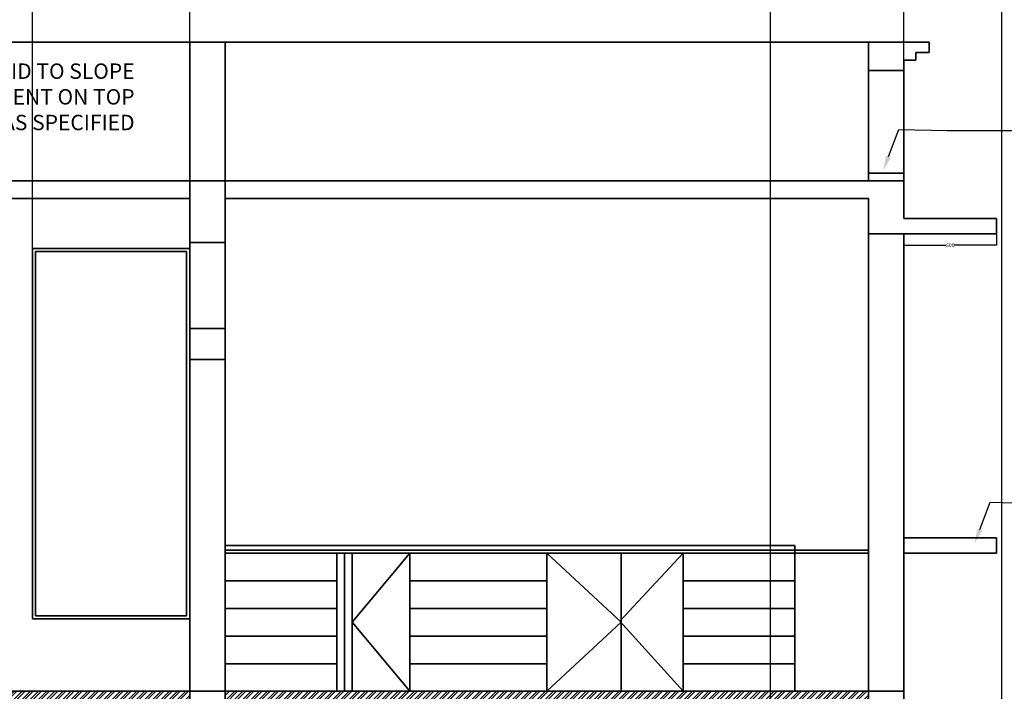
# Model space of a CAD drawing. Units: millimetres. Extents: x 1944 to 29915, y -10550 to 5909.
# Tile 20 of 24: x 19652 to 26040, y -5946 to -1584. Entities that reach past the tile are written whole.
import ezdxf
from ezdxf import colors
from ezdxf.entities.mleader import LeaderData, LeaderLine
from ezdxf.math import Vec2, Vec3

# ---------------------------------------------------------------- set-up
doc = ezdxf.new("R2010")
doc.units = ezdxf.units.MM
doc.header["$MEASUREMENT"] = 0
for name, color, linetype, lineweight in [('A-ANNO-DIMS', 2, 'Continuous', 18), ('A-ANNO-TEXT', 7, 'Continuous', 25), ('A-FLOR-PATT', 252, 'Continuous', 13), ('A-SECT', 7, 'Continuous', 35)]:
    doc.layers.add(name, color=color, linetype=linetype, lineweight=lineweight)
doc.styles.get("Standard").update_dxf_attribs({"font": 'arial.ttf'})
doc.dimstyles.get("Standard").update_dxf_attribs({"dimtxt": 25, "dimasz": 0.18, "dimexe": 0.18, "dimexo": 0.0625, "dimgap": 0.09, "dimtad": 0, "dimtih": 1, "dimtoh": 1, "dimdec": 0, "dimzin": 0, "dimdsep": 46, "dimtxsty": 'Standard', "dimcen": 0.09, "dimadec": 0, "dimazin": 0, "dimtfac": 1, "dimtdec": 0, "dimtofl": 0, "dimtmove": 0, "dimatfit": 3, "dimfxl": 1, "dimtolj": 1, "dimtzin": 0, "dimarcsym": 0})

# ---------------------------------------------------------------- blocks, each defined once
blk = doc.blocks.new('*D29')
at = {"layer": 'A-ANNO-DIMS', "color": 0, "lineweight": -2, "transparency": 16777216}
for p, q in [((25389.3, -2975.8), (25389.3, -3049.3)), ((25989.3, -2975.8), (25989.3, -3049.3)), ((25389.5, -3049.1), (25661.6, -3049.1)), ((25989.1, -3049.1), (25717, -3049.1))]:
    blk.add_line(p, q, dxfattribs=at)
at = {"layer": 'A-ANNO-DIMS', "color": 0, "transparency": 16777216}
for points in [[(25389.5, -3049.1), (25389.5, -3049.2), (25389.3, -3049.1)], [(25989.1, -3049.1), (25989.1, -3049.2), (25989.3, -3049.1)]]:
    blk.add_solid(points, dxfattribs=at)
at = {"layer": 'Defpoints', "color": 0, "transparency": 16777216}
for p in [(25389.3, -2975.8), (25989.3, -2975.8), (25989.3, -3049.1)]:
    blk.add_point(p, dxfattribs=at)
at = {"layer": 'A-ANNO-DIMS', "color": 0, "transparency": 16777216, "insert": (25689.3, -3049.1), "char_height": 25, "attachment_point": 5}
blk.add_mtext('\\A1;600', dxfattribs=at)
blk = doc.blocks.new('*D85')
at = {"layer": 'A-ANNO-DIMS', "color": 0, "lineweight": -2, "transparency": 16777216}
for p, q in [((6418.3, -1730.7), (6418.3, -395.6)), ((6418.5, -395.8), (15860.3, -395.8)), ((25389.1, -395.8), (15947.3, -395.8)), ((25389.3, -1846.5), (25389.3, -395.6))]:
    blk.add_line(p, q, dxfattribs=at)
at = {"layer": 'A-ANNO-DIMS', "color": 0, "transparency": 16777216}
for points in [[(6418.5, -395.7), (6418.5, -395.8), (6418.3, -395.8)], [(25389.1, -395.7), (25389.1, -395.8), (25389.3, -395.8)]]:
    blk.add_solid(points, dxfattribs=at)
at = {"layer": 'Defpoints', "color": 0, "transparency": 16777216}
for p in [(25389.3, -395.8), (6418.3, -1730.8), (25389.3, -1846.5)]:
    blk.add_point(p, dxfattribs=at)
at = {"layer": 'A-ANNO-DIMS', "color": 0, "transparency": 16777216, "insert": (15903.8, -395.8), "char_height": 25, "attachment_point": 5}
blk.add_mtext('\\A1;18971', dxfattribs=at)
blk = doc.blocks.new('*D91')
at = {"layer": 'A-ANNO-DIMS', "color": 0, "lineweight": -2, "transparency": 16777216}
for p, q in [((24524.3, -7516.2), (24524.3, -395.6)), ((24524.5, -395.8), (25238.1, -395.8)), ((26024.1, -395.8), (25310.5, -395.8)), ((26024.3, -7516.2), (26024.3, -395.6))]:
    blk.add_line(p, q, dxfattribs=at)
at = {"layer": 'A-ANNO-DIMS', "color": 0, "transparency": 16777216}
for points in [[(24524.5, -395.7), (24524.5, -395.8), (24524.3, -395.8)], [(26024.1, -395.7), (26024.1, -395.8), (26024.3, -395.8)]]:
    blk.add_solid(points, dxfattribs=at)
at = {"layer": 'Defpoints', "color": 0, "transparency": 16777216}
for p in [(26024.3, -395.8), (24524.3, -7516.2), (26024.3, -7516.2)]:
    blk.add_point(p, dxfattribs=at)
at = {"layer": 'A-ANNO-DIMS', "color": 0, "transparency": 16777216, "insert": (25274.3, -395.8), "char_height": 25, "attachment_point": 5}
blk.add_mtext('\\A1;1500', dxfattribs=at)
blk = doc.blocks.new('*D96')
at = {"layer": 'A-ANNO-DIMS', "color": 0, "lineweight": -2, "transparency": 16777216}
for p, q in [((19735.4, -3070.7), (19735.4, -395.6)), ((19735.6, -395.8), (20209.2, -395.8)), ((20755.3, -395.8), (20281.6, -395.8)), ((20755.4, -3070.7), (20755.4, -395.6))]:
    blk.add_line(p, q, dxfattribs=at)
at = {"layer": 'A-ANNO-DIMS', "color": 0, "transparency": 16777216}
for points in [[(19735.6, -395.7), (19735.6, -395.8), (19735.4, -395.8)], [(20755.3, -395.7), (20755.3, -395.8), (20755.4, -395.8)]]:
    blk.add_solid(points, dxfattribs=at)
at = {"layer": 'Defpoints', "color": 0, "transparency": 16777216}
for p in [(20755.4, -395.8), (19735.4, -3070.8), (20755.4, -3070.8)]:
    blk.add_point(p, dxfattribs=at)
at = {"layer": 'A-ANNO-DIMS', "color": 0, "transparency": 16777216, "insert": (20245.4, -395.8), "char_height": 25, "attachment_point": 5}
blk.add_mtext('\\A1;1020', dxfattribs=at)

msp = doc.modelspace()

# ---------------------------------------------------------------- hatches: boundary and pattern name
at = {"layer": 'A-FLOR-PATT'}
h = msp.add_hatch(dxfattribs=at)
h.set_pattern_fill('ANSI32', color=256, scale=100)
h.paths.add_polyline_path([(16977.828, -5945.752), (16977.828, -6073.852), (20755.45, -6073.852), (20755.45, -5945.752)])
h = msp.add_hatch(dxfattribs=at)
h.set_pattern_fill('ANSI32', color=256, scale=100)
h.paths.add_polyline_path([(25159.297, -5945.752), (20985.45, -5945.752), (20985.45, -6073.852), (25159.297, -6073.852)])

# ---------------------------------------------------------------- linework, layer by layer
at = {"layer": 'A-SECT'}
for p, q in [((16516.552, -1730.752), (20985.45, -1730.752)), ((20755.45, -1730.752), (20755.45, -2745.752)), ((20985.45, -1730.752), (20985.45, -2745.752)), ((20985.45, -1730.752), (25159.297, -1730.752)), ((25159.297, -1730.752), (25159.297, -2630.752)), ((25159.297, -1730.752), (25552.588, -1730.752)), ((25552.588, -1730.752), (25552.588, -1797.438)), ((25389.297, -1846.542), (25389.297, -2630.752)), ((25467.118, -1846.542), (25389.297, -1846.542)), ((25552.588, -1797.438), (25467.118, -1797.438)), ((25467.118, -1797.438), (25467.118, -1846.542)), ((25389.297, -1913.658), (25159.297, -1913.658)), ((25159.297, -2630.752), (25159.297, -2580.752)), ((25159.297, -2580.752), (25389.297, -2580.752)), ((12343.981, -2630.752), (25389.297, -2630.752)), ((25389.297, -2630.752), (25389.297, -2875.752)), ((16977.828, -2745.752), (20755.45, -2745.752)), ((20755.45, -2745.752), (20755.45, -5945.752)), ((20985.45, -2745.752), (25159.297, -2745.752)), ((25159.297, -2745.752), (25159.297, -2975.752)), ((25989.297, -2875.752), (25389.297, -2875.752)), ((25989.297, -2975.752), (25989.297, -2875.752)), ((25159.297, -2975.752), (25389.297, -2975.752)), ((25389.297, -2975.752), (25989.297, -2975.752)), ((25389.297, -2975.752), (25389.297, -5945.752)), ((20755.45, -3030.752), (20755.45, -5495.752)), ((20755.45, -3030.752), (20985.45, -3030.752)), ((19735.45, -5475.752), (19735.45, -3070.752)), ((19735.45, -3070.752), (20755.45, -3070.752)), ((19755.45, -5455.752), (19755.45, -3090.752)), ((19755.45, -3090.752), (20735.45, -3090.752)), ((20735.45, -3090.752), (20735.45, -5455.752)), ((20755.45, -3590.131), (20985.45, -3590.131)), ((20755.45, -3790.131), (20985.45, -3790.131)), ((25989.297, -4948.468), (25389.297, -4948.468)), ((25989.297, -5048.468), (25989.297, -4948.468)), ((20985.45, -4998.468), (24681.651, -4998.468)), ((20985.45, -5028.468), (25159.297, -5028.468)), ((24681.651, -4998.468), (24681.651, -5945.752)), ((20985.45, -5048.468), (25159.297, -5048.468)), ((20985.45, -5048.468), (21709.826, -5048.468)), ((21709.826, -5048.468), (21709.826, -5945.752)), ((21759.826, -5048.468), (21759.826, -5945.752)), ((21809.826, -5048.468), (21809.826, -5945.752)), ((21809.826, -5497.11), (22183.331, -5048.468)), ((22183.331, -5048.468), (22183.331, -5945.752)), ((23072.373, -5048.468), (23072.373, -5945.752)), ((23072.373, -5048.468), (23553.745, -5497.11)), ((23957.275, -5048.468), (23545.928, -5489.824)), ((23553.745, -5048.468), (23553.745, -5945.752)), ((23957.275, -5048.468), (23957.275, -5945.752)), ((25389.297, -5048.468), (25989.297, -5048.468)), ((20985.45, -5227.925), (21709.826, -5227.925)), ((22183.331, -5227.925), (23072.373, -5227.925)), ((23957.275, -5227.925), (24681.651, -5227.925)), ((20985.45, -5407.382), (21709.826, -5407.382)), ((22183.331, -5407.382), (23072.373, -5407.382)), ((23957.275, -5407.382), (24681.651, -5407.382)), ((20755.45, -5475.752), (19735.45, -5475.752)), ((20735.45, -5455.752), (19755.45, -5455.752)), ((23545.928, -5489.824), (23957.275, -5945.752)), ((22183.331, -5945.752), (21809.826, -5497.11)), ((23553.745, -5497.11), (23072.373, -5945.752)), ((20985.45, -5586.838), (21709.826, -5586.838)), ((22183.331, -5586.838), (23072.373, -5586.838)), ((23957.275, -5586.838), (24681.651, -5586.838)), ((20985.45, -5766.295), (21709.826, -5766.295)), ((22183.331, -5766.295), (23072.373, -5766.295)), ((23957.275, -5766.295), (24681.651, -5766.295)), ((20755.45, -5945.752), (16977.828, -5945.752)), ((20985.45, -5945.752), (21709.826, -5945.752)), ((23957.275, -5945.752), (24681.651, -5945.752))]:
    msp.add_line(p, q, dxfattribs=at)
for points in [[(20985.45, -2745.752), (20985.45, -5945.752), (25159.297, -5945.752), (25159.297, -2745.752)], [(25389.297, -5945.752), (25389.297, -6305.752), (25159.297, -6305.752), (25159.297, -5945.752), (25389.297, -5945.752)]]:
    msp.add_lwpolyline(points, dxfattribs=at)
msp.add_lwpolyline([(20755.45, -5945.752), (20985.45, -5945.752), (20985.45, -6305.752), (20755.45, -6305.752)], close=True, dxfattribs=at)

# ---------------------------------------------------------------- dimensions: what is measured, and where the dimension line sits
at = {"layer": 'A-ANNO-DIMS'}
for base, p1, p2, override, picture, middle in [((25389.297, -395.752), (6418.315, -1730.752), (25389.297, -1846.542), {"dimdec": 0, "dimlfac": 1, "dimrnd": 0, "dimzin": 0, "dimdsep": 46, "dimlunit": 2}, '*D85', (15903.806, -395.752)), ((20755.45, -395.752), (19735.45, -3070.752), (20755.45, -3070.752), {"dimdec": 0, "dimlfac": 1, "dimrnd": 0, "dimzin": 0, "dimdsep": 46, "dimlunit": 2}, '*D96', (20245.45, -395.752)), ((26024.297, -395.752), (24524.297, -7516.218), (26024.297, -7516.218), {"dimdec": 0, "dimlfac": 1, "dimrnd": 0, "dimzin": 0, "dimdsep": 46, "dimlunit": 2}, '*D91', (25274.297, -395.752)), ((25989.297, -3049.123), (25389.297, -2975.752), (25989.297, -2975.752), {"dimclrd": 0, "dimclre": 0, "dimclrt": 0}, '*D29', (25689.297, -3049.123))]:
    dim = msp.add_linear_dim(base=base, p1=p1, p2=p2, dimstyle='Standard', override=override, dxfattribs=at)
    dim.commit()
    dim.dimension.update_dxf_attribs({"geometry": picture, "text_midpoint": middle})

# ---------------------------------------------------------------- leaders
at = {"layer": 'A-ANNO-TEXT'}
ml = msp.add_multileader_mtext('Standard', dxfattribs=at)
ml.set_content('RCC ROOF SLAB LAID TO SLOPE \\PWITH WATER  PROOFING TREATMENT ON TOP \\PAS SPECIFIED', color=256)
ml.set_leader_properties()
ml.build(insert=Vec2(0, 0))
ml.multileader.update_dxf_attribs({"dogleg_length": 568.936, "arrow_head_size": 100})
ctx = ml.context
ctx.base_point, ctx.char_height, ctx.arrow_head_size, ctx.landing_gap_size, ctx.plane_origin = Vec3(17215.618, -1919.582), 100, 100, 0.09, Vec3(17085.053, -2367.807)
ctx.text_align_type = 2
notes = []
notes.append((ctx, [(0, (1, 1, 0), (16646.682, -1919.582), (1, 0), 568.936, [(0, [(16669.038, -2630.752), (16677.34, -2324.48)], 0, [])])]))
ctx.mtext.insert, ctx.mtext.alignment, ctx.mtext.flow_direction = Vec3(20397.632, -1868.729), 3, 5
ml = msp.add_multileader_mtext('Standard', dxfattribs=at)
ml.set_content('PCC BENCHING', color=256)
ml.set_leader_properties()
ml.build(insert=Vec2(0, 0))
ml.multileader.update_dxf_attribs({"dogleg_length": 568.936, "arrow_head_size": 100})
ctx = ml.context
ctx.base_point, ctx.char_height, ctx.arrow_head_size, ctx.landing_gap_size, ctx.plane_origin = Vec3(26238.375, -2303.899), 100, 100, 0.09, Vec3(25669.439, -2303.899)
ctx.text_align_type = 2
notes.append((ctx, [(0, (1, 1, 0), (25669.439, -2303.899), (1, 0), 568.936, [(0, [(25253.425, -2566.843), (25356.203, -2296.612)], 0, [])])]))
ctx.mtext.insert, ctx.mtext.alignment, ctx.mtext.flow_direction = Vec3(27290.102, -2253.046), 3, 5
ml = msp.add_multileader_mtext('Standard', dxfattribs=at)
ml.set_content('COOLER RESTY', color=256)
ml.set_leader_properties()
ml.build(insert=Vec2(0, 0))
ml.multileader.update_dxf_attribs({"dogleg_length": 568.936, "arrow_head_size": 100})
ctx = ml.context
ctx.base_point, ctx.char_height, ctx.arrow_head_size, ctx.landing_gap_size, ctx.plane_origin = Vec3(26831.222, -4724.765), 100, 100, 0.09, Vec3(26262.286, -4724.765)
ctx.text_align_type = 2
notes.append((ctx, [(0, (1, 1, 0), (26262.286, -4724.765), (1, 0), 568.936, [(0, [(25846.272, -4987.709), (25949.05, -4717.477)], 0, [])])]))
ctx.mtext.insert, ctx.mtext.alignment, ctx.mtext.flow_direction = Vec3(27917.806, -4673.912), 3, 5
for ctx, leaders in notes:
    for number, flags, end, landing, length, lines in leaders:
        leader = LeaderData()
        leader.index, (leader.has_last_leader_line, leader.has_dogleg_vector, leader.attachment_direction) = number, flags
        leader.last_leader_point, leader.dogleg_vector, leader.dogleg_length = Vec3(end), Vec3(landing), length
        for number, points, colour, breaks in lines:
            line = LeaderLine()
            line.index, line.vertices, line.color, line.breaks = number, Vec3.list(points), colors.encode_raw_color(colour), breaks
            leader.lines.append(line)
        ctx.leaders.append(leader)

doc.saveas('drawing.dxf')
